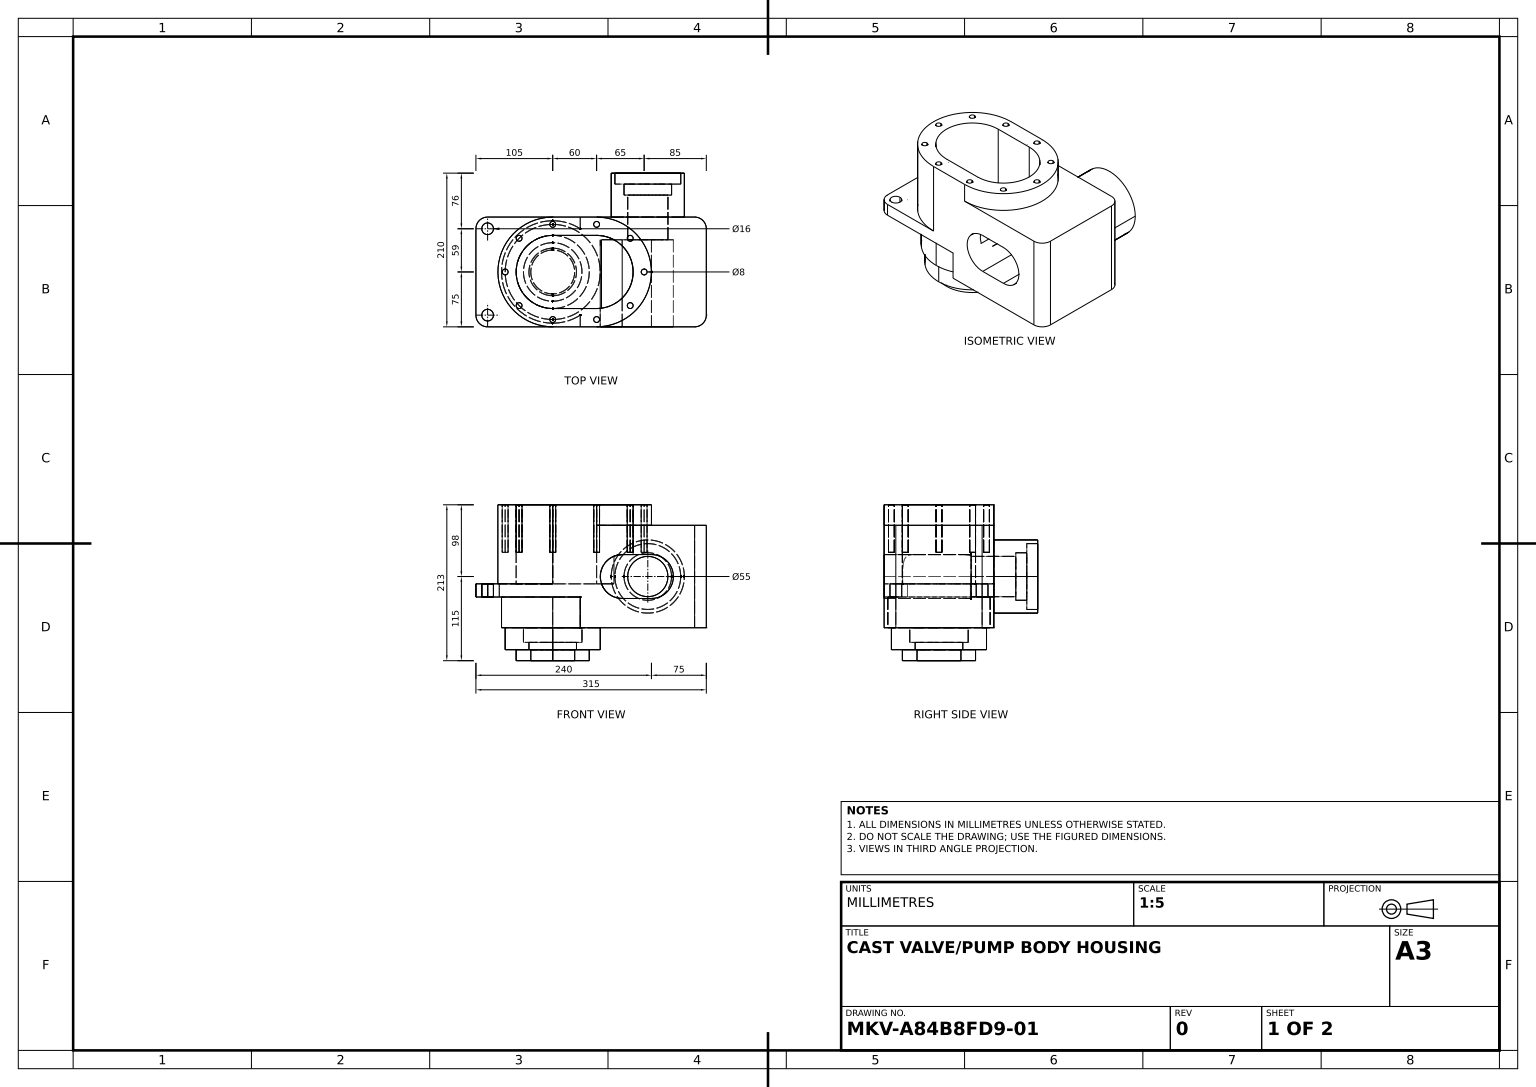
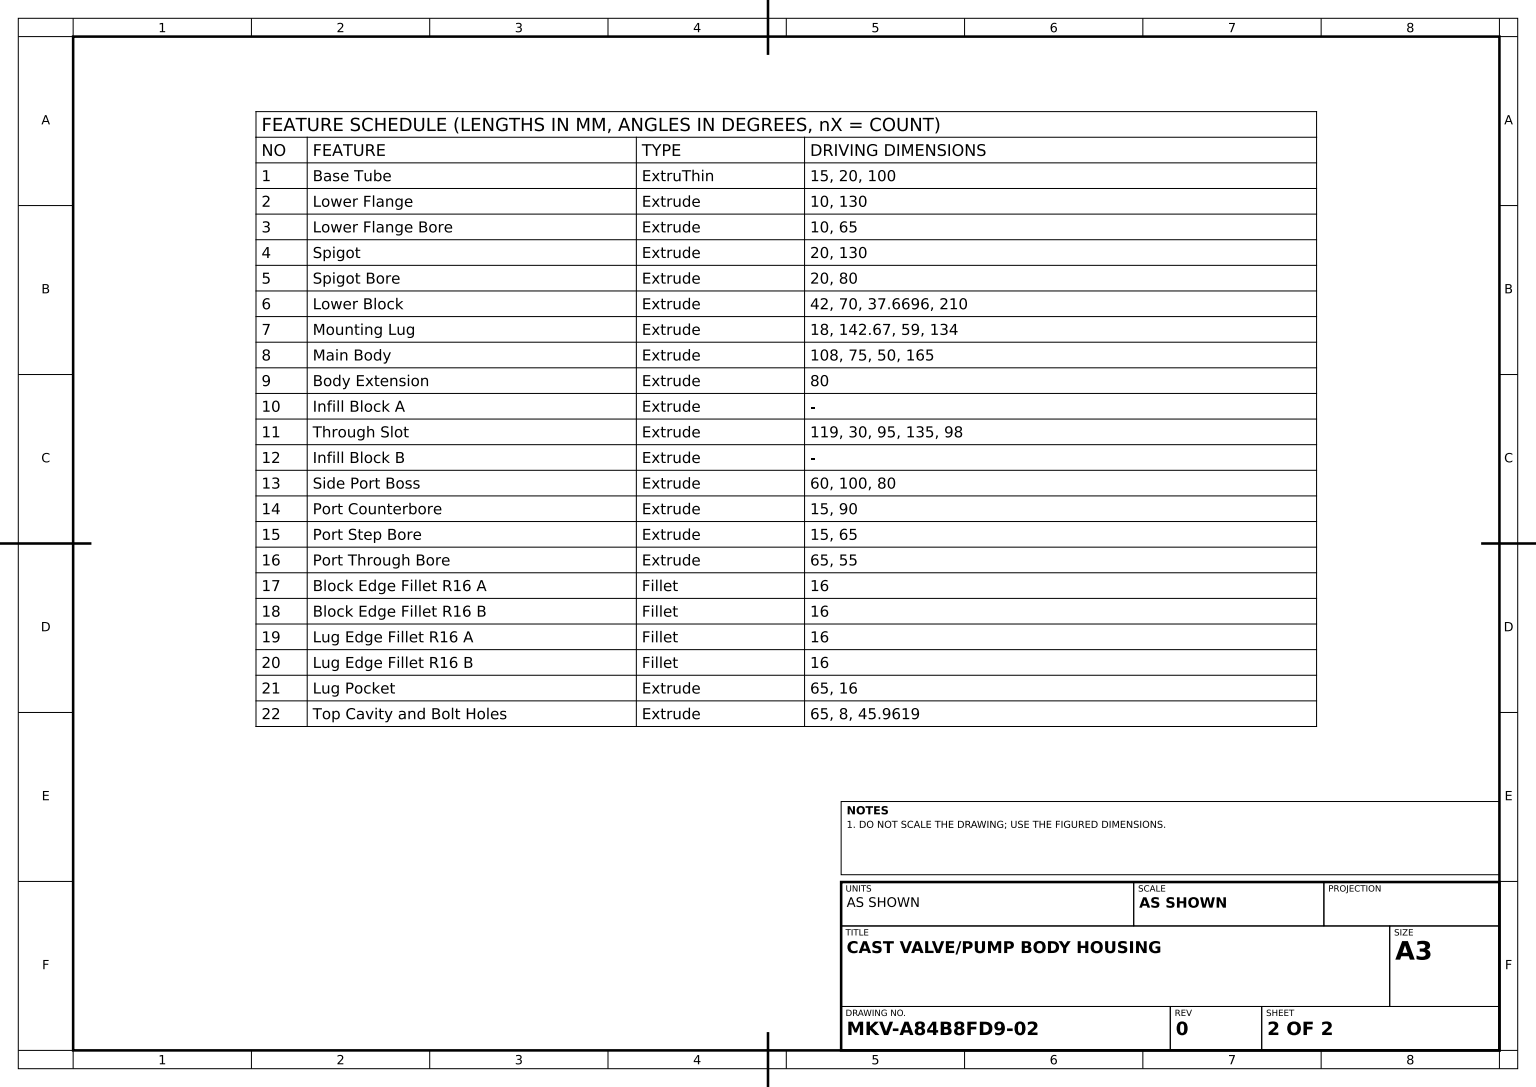
SolidWorks part; units mm, degrees
material "Plain Carbon Steel"
ref_plane "Front Plane" through (0, 0, 0) normal (0, 0, 1) x (1, 0, 0)
ref_plane "Top Plane" through (0, 0, 0) normal (0, 1, 0) x (1, 0, 0)
ref_plane "Right Plane" through (0, 0, 0) normal (1, 0, 0) x (0, 0, -1)
sketch "Base Tube Sketch" plane through (0, 0, 0) normal (0, 1, 0) x (1, 0, 0)
  circle A0 centre (0, 0) radius 50
  dimension "D1" = 100
extrude "Base Tube" add sketch "Base Tube Sketch" along normal blind 15 thin thin type one direction reverse wall 20
sketch "Lower Flange Sketch" plane through (0, 15, 0) normal (0, 1, 0) x (1, 0, 0)
  circle A0 centre (0, 0) radius 65
  dimension "D1" = 130
extrude "Lower Flange" add sketch "Lower Flange Sketch" along normal blind 10
sketch "Lower Flange Bore Sketch" plane through (0, 25, 0) normal (0, 1, 0) x (1, 0, 0)
  circle A0 centre (0, 0) radius 32.5
  dimension "D1" = 65
extrude "Lower Flange Bore" cut sketch "Lower Flange Bore Sketch" against normal blind 10
sketch "Spigot Sketch" plane through (0, 25, 0) normal (0, 1, 0) x (1, 0, 0)
  circle A0 centre (0, 0) radius 65
  dimension "D1" = 130
extrude "Spigot" add sketch "Spigot Sketch" along normal blind 20
sketch "Spigot Bore Sketch" plane through (0, 45, 0) normal (0, 1, 0) x (1, 0, 0)
  circle A0 centre (0, 0) radius 40
  dimension "D1" = 80
extrude "Spigot Bore" cut sketch "Spigot Bore Sketch" against normal blind 20
sketch "Lower Block Sketch" plane through (0, 45, 0) normal (0, 1, 0) x (1, 0, 0)
  line L1 (37.6696, 59) -> (210, 59)
  line L2 (210, 59) -> (210, -59)
  line L3 (210, -59) -> (37.6696, -59)
  arc A0 (37.6696, 59) -> (37.6696, -59) centre (0, 0) ccw
  circle A1 centre (0, 0) radius 40 construction
  dimension "D1" = 70
  dimension "D2" = 37.6696
  dimension "D3" = 210
extrude "Lower Block" add sketch "Lower Block Sketch" along normal blind 42
sketch "Mounting Lug Sketch" plane through (0, 87, 0) normal (0, 1, 0) x (1, 0, 0)
  line L0 (37.6696, -59) -> (210, -59) construction
  line L2 (-105, 0) -> (-105, 75)
  line L3 (-105, 75) -> (210, 75)
  line L4 (210, 75) -> (210, -75)
  line L5 (210, -75) -> (-105, -75)
  line L6 (-105, -75) -> (-105, 0)
  dimension "D1" = 142.6696
  dimension "D2" = 59
  dimension "D3" = 134
extrude "Mounting Lug" add sketch "Mounting Lug Sketch" along normal blind 18
sketch "Main Body Sketch" plane through (0, 105, 0) normal (0, 1, 0) x (1, 0, 0)
  line L1 (0, 75) -> (60, 75)
  line L2 (-105, 75) -> (-105, -75) construction
  line L3 (0, -75) -> (60, -75)
  line L7 (0, 50) -> (60, 50)
  line L8 (0, -50) -> (60, -50)
  arc A0 (0, 75) -> (0, -75) centre (0, 0) ccw
  arc A1 (0, 50) -> (0, -50) centre (0, 0) ccw
  arc A2 (60, 50) -> (60, -50) centre (60, 0) cw
  arc A3 (60, 75) -> (60, -75) centre (60, 0) cw
  dimension "D1" = 75
  dimension "D2" = 50
  dimension "D3" = 165
extrude "Main Body" add sketch "Main Body Sketch" along normal blind 108
sketch "Body Extension Sketch" plane through (0, 105, 0) normal (0, 1, 0) x (1, 0, 0)
  line L0 (60, 75) -> (210, 75)
  line L1 (210, 75) -> (210, -75)
  line L2 (210, -75) -> (60, -75)
  arc A0 (60, 75) -> (60, -75) centre (60, 0) cw
extrude "Body Extension" add sketch "Body Extension Sketch" along normal blind 80
sketch "Infill Block A Sketch" plane through (0, 0, 59) normal (0, 0, 1) x (1, 0, 0)
  line L0 (37.6696, 87) -> (210, 87)
  line L1 (210, 87) -> (210, 45)
  line L2 (210, 45) -> (37.6696, 45)
  line L3 (37.6696, 45) -> (37.6696, 87)
extrude "Infill Block A" add sketch "Infill Block A Sketch" along normal up to vertex (16 mm away)
sketch "Through Slot Sketch" plane through (0, 0, 75) normal (0, 0, 1) x (1, 0, 0)
  line L0 (0, 213) -> (0, 105) construction
  line L1 (0, 213) -> (60, 213) construction
  line L3 (95, 145) -> (135, 145)
  line L4 (95, 85) -> (135, 85)
  arc A0 (135, 85) -> (135, 145) centre (135, 115) ccw
  arc A1 (95, 145) -> (95, 85) centre (95, 115) ccw
  dimension "D1" = 30
  dimension "D2" = 95
  dimension "D3" = 135
  dimension "D4" = 98
extrude "Through Slot" cut sketch "Through Slot Sketch" against normal blind 119
sketch "Infill Block B Sketch" plane through (0, 0, -59) normal (0, 0, -1) x (-1, 0, 0)
  line L0 (-210, 87) -> (-37.6696, 87)
  line L1 (-37.6696, 87) -> (-37.6696, 45)
  line L2 (-37.6696, 45) -> (-210, 45)
  line L3 (-210, 45) -> (-210, 87)
extrude "Infill Block B" add sketch "Infill Block B Sketch" along normal up to vertex (16 mm away)
sketch "Side Port Boss Sketch" plane through (0, 0, -75) normal (0, 0, -1) x (-1, 0, 0)
  line L0 (-210, 115) -> (-130, 115)
  line L1 (-210, 185) -> (-210, 45) construction
  circle A0 centre (-130, 115) radius 50
  dimension "D1" = 100
  dimension "D2" = 80
extrude "Side Port Boss" add sketch "Side Port Boss Sketch" along normal blind 60
sketch "Port Counterbore Sketch" plane through (0, 0, -135) normal (0, 0, -1) x (-1, 0, 0)
  circle A0 centre (-130, 115) radius 45
  dimension "D1" = 90
extrude "Port Counterbore" cut sketch "Port Counterbore Sketch" against normal blind 15
sketch "Port Step Bore Sketch" plane through (0, 0, -120) normal (0, 0, -1) x (-1, 0, 0)
  circle A0 centre (-130, 115) radius 32.5
  dimension "D1" = 65
extrude "Port Step Bore" cut sketch "Port Step Bore Sketch" against normal blind 15
sketch "Port Through Bore Sketch" plane through (0, 0, -105) normal (0, 0, -1) x (-1, 0, 0)
  circle A0 centre (-130, 115) radius 27.5
  dimension "D1" = 55
extrude "Port Through Bore" cut sketch "Port Through Bore Sketch" against normal blind 65
fillet "Block Edge Fillet R16 A" radius 16 1 edges at (210, 115, 75)
fillet "Block Edge Fillet R16 B" radius 16 1 edges at (210, 115, -75)
fillet "Lug Edge Fillet R16 A" radius 16 1 edges at (-105, 96, 75)
fillet "Lug Edge Fillet R16 B" radius 16 1 edges at (-105, 96, -75)
sketch "Lug Pocket Sketch" plane through (0, 105, 0) normal (0, 1, 0) x (1, 0, 0)
  circle A0 centre (-89, 59) radius 8
  circle A1 centre (-89, -59) radius 8
  dimension "D1" = 16
extrude "Lug Pocket" cut sketch "Lug Pocket Sketch" against normal blind 65
sketch "Top Cavity and Bolt Holes Sketch" plane through (0, 213, 0) normal (0, 1, 0) x (1, 0, 0)
  line L0 (4, 65) -> (56, 65)
  line L1 (4, -65) -> (56, -65)
  arc A0 (-3.9981, 64.8769) -> (-43.0478, 48.702) centre (0, 0) ccw
  arc A1 (63.9981, -64.8769) -> (103.0478, -48.702) centre (60, 0) ccw
  circle A2 centre (0, 65) radius 4
  circle A3 centre (60, 65) radius 4
  circle A4 centre (-65, 0) radius 4
  circle A5 centre (0, -65) radius 4
  circle A6 centre (60, -65) radius 4
  circle A7 centre (125, 0) radius 4
  circle A8 centre (105.9619, 45.9619) radius 4
  circle A9 centre (105.9619, -45.9619) radius 4
  circle A10 centre (-45.9619, -45.9619) radius 4
  circle A11 centre (-45.9619, 45.9619) radius 4
  arc A12 (-48.702, 43.0478) -> (-64.8769, 3.9981) centre (0, 0) ccw
  arc A13 (103.0478, 48.702) -> (63.9981, 64.8769) centre (60, 0) ccw
  arc A14 (124.8769, 3.9981) -> (108.702, 43.0478) centre (60, 0) ccw
  arc A15 (108.702, -43.0478) -> (124.8769, -3.9981) centre (60, 0) ccw
  arc A16 (-64.8769, -3.9981) -> (-48.702, -43.0478) centre (0, 0) ccw
  arc A17 (-43.0478, -48.702) -> (-3.9981, -64.8769) centre (0, 0) ccw
  dimension "D1" = 65
  dimension "D2" = 8
  dimension "D3" = 45.9619
extrude "Top Cavity and Bolt Holes" cut sketch "Top Cavity and Bolt Holes Sketch" against normal blind 65 contours A4 | A3 | A8 | A7 | A9 | A10 | A11 | A2 | A6 | A5
